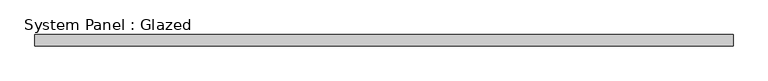
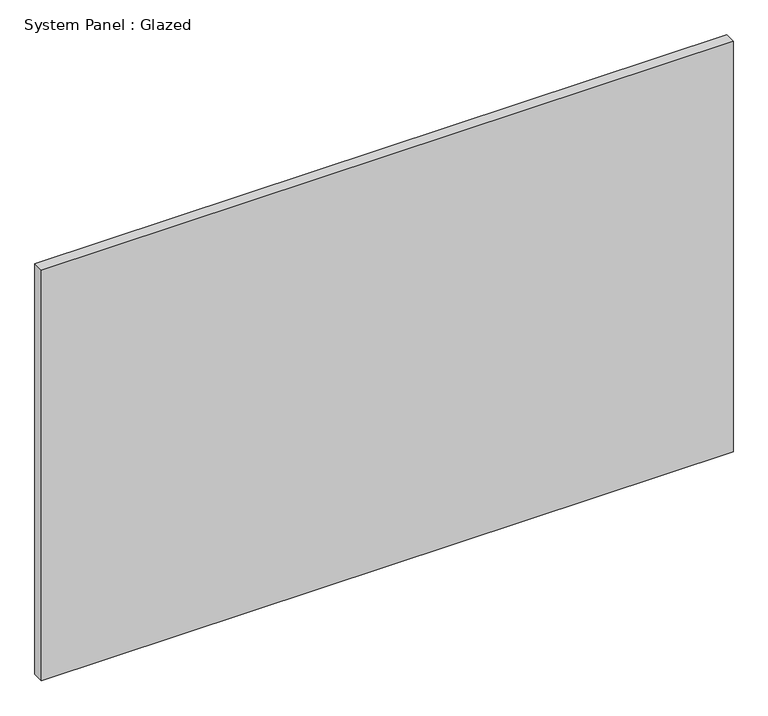
"""IFC4 building model written with IfcOpenShell, lengths in millimetres: plate geometry, System Panel : Glazed."""

from ifc_helpers import new_model, si_unit, origin, origin_with_axes, place, context, project, spatial, polyline, outline, extrude, source, transform, mapped, element, save


def system_panel_glazed_3160786d(model_context):
    return source(origin(), model_context, "Body", "SweptSolid", [
        extrude(outline(polyline([(780.9146696, 19.05), (-780.9146696, 19.05), (-780.9146696, 44.45), (780.9146696, 44.45), (780.9146696, 19.05)])), origin_with_axes(), (0.0, 0.0, 1.0), 979.2807647),
    ])


if __name__ == "__main__":
    model = new_model("IFC4")
    model_context = context("Model", 3, world=origin())
    ifc_project = project(units=[si_unit("LENGTHUNIT", "METRE", prefix="MILLI")], contexts=[model_context])
    site = spatial("IfcSite", under=ifc_project)
    building = spatial("IfcBuilding", under=site)
    placement = place(None, origin())
    system_panel_glazed_shape = system_panel_glazed_3160786d(model_context)
    element("IfcPlate", 1, ObjectType="System Panel : Glazed", at=placement, inside=building, context=model_context, shape_type="MappedRepresentation", body=[
        mapped(system_panel_glazed_shape, transform((0.0, 0.0, 0.0), x_axis=(1.0, 0.0, 0.0), y_axis=(0.0, 1.0, 0.0), z_axis=(0.0, 0.0, 1.0))),
    ])
    save(model, "model.ifc")

# Revit data of these elements
# Type "System Panel : Glazed"
#   Construction Type Id = "GSP4R"
#   Analytic Construction = "1/8 in Pilkington single glazing"
#   Visual Light Transmittance = 0.9
#   Solar Heat Gain Coefficient = 0.86
#   Heat Transfer Coefficient (U) = 1.18115 BTU/(h·ft²·°F)
#   Define Thermal Properties by = 1
# Element 1 (IfcPlate, "System Panel : Glazed")
#   Materials on its faces: "Glass"
# Materials
#   "Glass": class "Glass", colour RGB 0 128 192, transparency 0.75, Description = "Soda Lime Glass", Cost = 0
